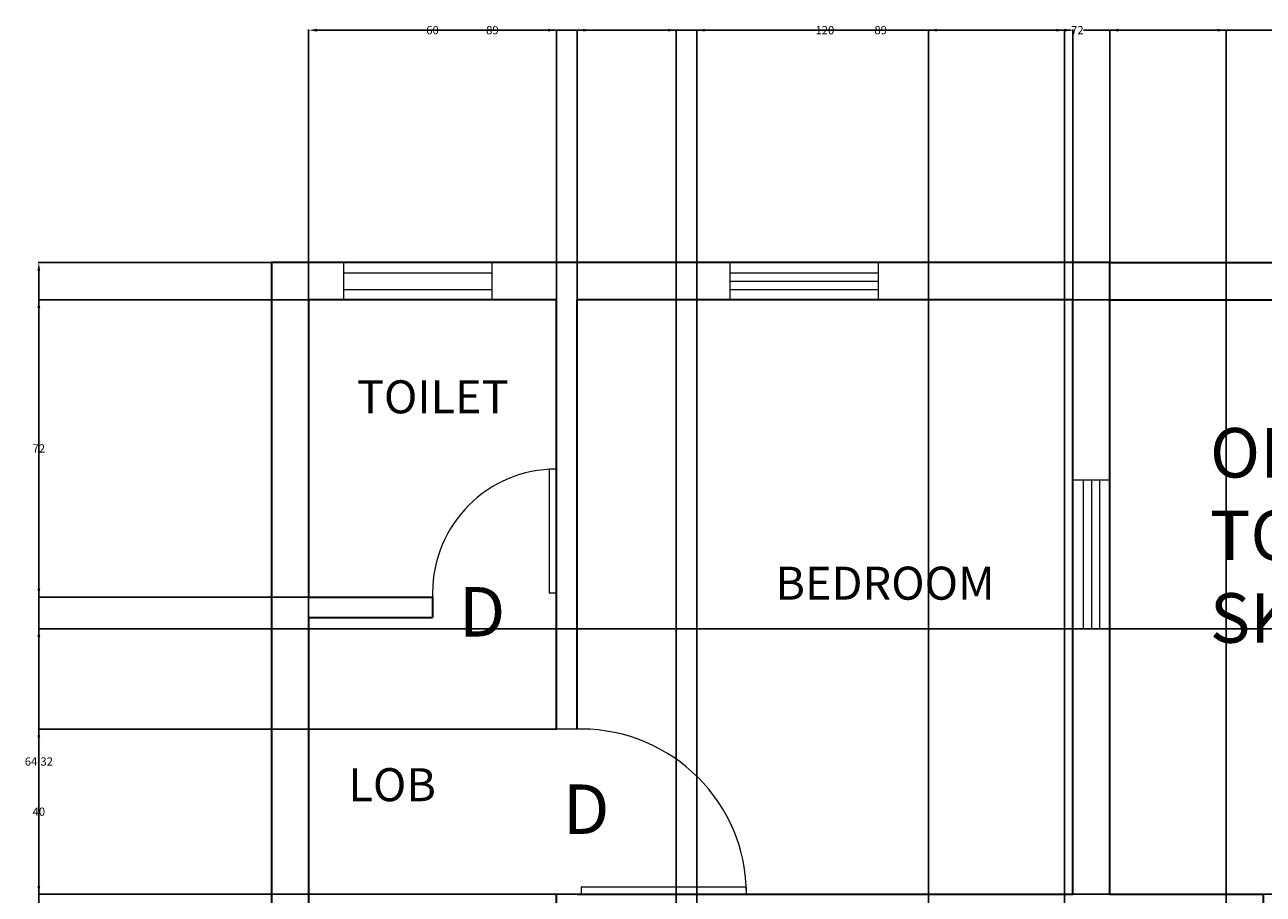
# Model space of a CAD drawing. Units: inches. Extents: x 190 to 836, y -241 to 999.
# Tile 7 of 9: x 191 to 491, y 789 to 999. Entities that reach past the tile are written whole.
import ezdxf

# ---------------------------------------------------------------- set-up
doc = ezdxf.new("R2010")
doc.units = ezdxf.units.IN
doc.header["$MEASUREMENT"] = 0
for name, color, linetype, lineweight in [('A-ANNO-DIMS', 2, 'Continuous', 18), ('A-ANNO-TEXT', 7, 'Continuous', 18), ('A-AREA-IDEN', 7, 'Continuous', 18), ('A-DOOR', 3, 'Continuous', 18), ('A-GLAZ', 4, 'Continuous', 18), ('A-WALL', 7, 'Continuous', 35)]:
    doc.layers.add(name, color=color, linetype=linetype, lineweight=lineweight)
doc.styles.get("Standard").update_dxf_attribs({"font": 'arial.ttf'})
doc.dimstyles.get("Standard").update_dxf_attribs({"dimtxt": 2, "dimasz": 2, "dimexe": 0.18, "dimexo": 0.0625, "dimgap": 0.09, "dimtad": 0, "dimtih": 1, "dimtoh": 1, "dimdec": 0, "dimzin": 0, "dimdsep": 46, "dimlunit": 3, "dimtxsty": 'Standard', "dimcen": 0.09, "dimadec": 0, "dimazin": 0, "dimtfac": 1, "dimtdec": 0, "dimtofl": 0, "dimtmove": 0, "dimatfit": 3, "dimfxl": 1, "dimtolj": 1, "dimtzin": 0, "dimarcsym": 0})

# ---------------------------------------------------------------- blocks, each defined once
blk = doc.blocks.new('*U2')
for p, q in [((0, 0), (0, 6)), ((40, 0), (40, 6))]:
    blk.add_line(p, q)
blk.add_lwpolyline([(0, 0), (0, -40), (1.75, -40), (1.75, 0)], close=True)
blk.add_arc((0, 0), 40, 270, 360)
blk = doc.blocks.new('*U3')
for p, q in [((-30, 0), (-30, -6)), ((0, 0), (0, -6))]:
    blk.add_line(p, q)
blk.add_lwpolyline([(0, 0), (0, 30), (-1.75, 30), (-1.75, 0)], close=True)
blk.add_arc((0, 0), 30, 90, 180)
blk = doc.blocks.new('WIN-36IN-9IN-3LINE')
for p, q in [((2.5, 36), (2.5, 0)), ((4.5, 36), (4.5, 0)), ((6.5, 36), (6.5, 0))]:
    blk.add_line(p, q)
blk.add_lwpolyline([(0, 0), (9, 0), (9, 36), (0, 36)], close=True)
blk = doc.blocks.new('WIN-36IN-9IN-2LINE')
for p, q in [((0, 6.5), (36, 6.5)), ((0, 2.5), (36, 2.5))]:
    blk.add_line(p, q)
blk.add_lwpolyline([(36, 0), (36, 9), (0, 9), (0, 0)], close=True)
blk = doc.blocks.new('*D17')
at = {"layer": 'A-ANNO-DIMS', "color": 0, "lineweight": -2, "transparency": 16777216}
for p, q in [((250.38, 941.53), (193.96, 941.53)), ((194.14, 939.53), (194.14, 380.14)), ((194.14, -181.47), (194.14, 377.92)), ((447.38, -183.47), (193.96, -183.47))]:
    blk.add_line(p, q, dxfattribs=at)
at = {"layer": 'A-ANNO-DIMS', "color": 0, "transparency": 16777216}
for points in [[(193.8, 939.53), (194.47, 939.53), (194.14, 941.53)], [(193.8, -181.47), (194.47, -181.47), (194.14, -183.47)]]:
    blk.add_solid(points, dxfattribs=at)
at = {"layer": 'Defpoints', "color": 0, "transparency": 16777216}
for p in [(194.14, 941.53), (250.44, 941.53), (447.44, -183.47)]:
    blk.add_point(p, dxfattribs=at)
at = {"layer": 'A-ANNO-DIMS', "color": 0, "transparency": 16777216, "insert": (194.14, 379.03), "char_height": 2, "attachment_point": 5}
blk.add_mtext('\\A1;1125', dxfattribs=at)
blk = doc.blocks.new('*D19')
at = {"layer": 'A-ANNO-DIMS', "color": 0, "lineweight": -2, "transparency": 16777216}
for p, q in [((453.44, 941.59), (453.44, 998.02)), ((455.44, 997.84), (511.24, 997.84)), ((571.44, 997.84), (515.64, 997.84)), ((573.44, 941.59), (573.44, 998.02))]:
    blk.add_line(p, q, dxfattribs=at)
at = {"layer": 'A-ANNO-DIMS', "color": 0, "transparency": 16777216}
for points in [[(455.44, 998.17), (455.44, 997.5), (453.44, 997.84)], [(571.44, 998.17), (571.44, 997.5), (573.44, 997.84)]]:
    blk.add_solid(points, dxfattribs=at)
at = {"layer": 'Defpoints', "color": 0, "transparency": 16777216}
for p in [(573.44, 997.84), (453.44, 941.53), (573.44, 941.53)]:
    blk.add_point(p, dxfattribs=at)
at = {"layer": 'A-ANNO-DIMS', "color": 0, "transparency": 16777216, "insert": (513.44, 997.84), "char_height": 2, "attachment_point": 5}
blk.add_mtext('\\A1;120', dxfattribs=at)
blk = doc.blocks.new('*D22')
at = {"layer": 'A-ANNO-DIMS', "color": 0, "lineweight": -2, "transparency": 16777216}
for p, q in [((259.44, 932.59), (259.44, 998.02)), ((261.44, 997.84), (287.92, 997.84)), ((317.44, 997.84), (290.97, 997.84)), ((319.44, 932.59), (319.44, 998.02))]:
    blk.add_line(p, q, dxfattribs=at)
at = {"layer": 'A-ANNO-DIMS', "color": 0, "transparency": 16777216}
for points in [[(261.44, 998.17), (261.44, 997.5), (259.44, 997.84)], [(317.44, 998.17), (317.44, 997.5), (319.44, 997.84)]]:
    blk.add_solid(points, dxfattribs=at)
at = {"layer": 'Defpoints', "color": 0, "transparency": 16777216}
for p in [(319.44, 997.84), (259.44, 932.53), (319.44, 932.53)]:
    blk.add_point(p, dxfattribs=at)
at = {"layer": 'A-ANNO-DIMS', "color": 0, "transparency": 16777216, "insert": (289.44, 997.84), "char_height": 2, "attachment_point": 5}
blk.add_mtext('\\A1;60', dxfattribs=at)
blk = doc.blocks.new('*D23')
at = {"layer": 'A-ANNO-DIMS', "color": 0, "lineweight": -2, "transparency": 16777216}
for p, q in [((324.44, 932.59), (324.44, 998.02)), ((326.44, 997.84), (382.24, 997.84)), ((442.44, 997.84), (386.64, 997.84)), ((444.44, 932.59), (444.44, 998.02))]:
    blk.add_line(p, q, dxfattribs=at)
at = {"layer": 'A-ANNO-DIMS', "color": 0, "transparency": 16777216}
for points in [[(326.44, 998.17), (326.44, 997.5), (324.44, 997.84)], [(442.44, 998.17), (442.44, 997.5), (444.44, 997.84)]]:
    blk.add_solid(points, dxfattribs=at)
at = {"layer": 'Defpoints', "color": 0, "transparency": 16777216}
for p in [(444.44, 997.84), (324.44, 932.53), (444.44, 932.53)]:
    blk.add_point(p, dxfattribs=at)
at = {"layer": 'A-ANNO-DIMS', "color": 0, "transparency": 16777216, "insert": (384.44, 997.84), "char_height": 2, "attachment_point": 5}
blk.add_mtext('\\A1;120', dxfattribs=at)
blk = doc.blocks.new('*D24')
at = {"layer": 'A-ANNO-DIMS', "color": 0, "lineweight": -2, "transparency": 16777216}
for p, q in [((259.38, 932.53), (193.96, 932.53)), ((194.14, 930.53), (194.14, 897.63)), ((194.14, 862.53), (194.14, 895.44)), ((259.38, 860.53), (193.96, 860.53))]:
    blk.add_line(p, q, dxfattribs=at)
at = {"layer": 'A-ANNO-DIMS', "color": 0, "transparency": 16777216}
for points in [[(193.8, 930.53), (194.47, 930.53), (194.14, 932.53)], [(193.8, 862.53), (194.47, 862.53), (194.14, 860.53)]]:
    blk.add_solid(points, dxfattribs=at)
at = {"layer": 'Defpoints', "color": 0, "transparency": 16777216}
for p in [(194.14, 932.53), (259.44, 932.53), (259.44, 860.53)]:
    blk.add_point(p, dxfattribs=at)
at = {"layer": 'A-ANNO-DIMS', "color": 0, "transparency": 16777216, "insert": (194.14, 896.53), "char_height": 2, "attachment_point": 5}
blk.add_mtext('\\A1;72', dxfattribs=at)
blk = doc.blocks.new('*D25')
at = {"layer": 'A-ANNO-DIMS', "color": 0, "lineweight": -2, "transparency": 16777216}
for p, q in [((444.5, 932.53), (832.94, 932.53)), ((832.76, 930.53), (832.76, 861.63)), ((832.76, 790.53), (832.76, 859.44)), ((444.5, 788.53), (832.94, 788.53))]:
    blk.add_line(p, q, dxfattribs=at)
at = {"layer": 'A-ANNO-DIMS', "color": 0, "transparency": 16777216}
for points in [[(832.43, 930.53), (833.1, 930.53), (832.76, 932.53)], [(832.43, 790.53), (833.1, 790.53), (832.76, 788.53)]]:
    blk.add_solid(points, dxfattribs=at)
at = {"layer": 'Defpoints', "color": 0, "transparency": 16777216}
for p in [(444.44, 932.53), (832.76, 932.53), (444.44, 788.53)]:
    blk.add_point(p, dxfattribs=at)
at = {"layer": 'A-ANNO-DIMS', "color": 0, "transparency": 16777216, "insert": (832.76, 860.53), "char_height": 2, "attachment_point": 5}
blk.add_mtext('\\A1;144', dxfattribs=at)
blk = doc.blocks.new('*D26')
at = {"layer": 'A-ANNO-DIMS', "color": 0, "lineweight": -2, "transparency": 16777216}
for p, q in [((409.55, 683.59), (409.55, 998.02)), ((411.55, 997.84), (444.05, 997.84)), ((479.55, 997.84), (447.06, 997.84)), ((481.55, 683.59), (481.55, 998.02))]:
    blk.add_line(p, q, dxfattribs=at)
at = {"layer": 'A-ANNO-DIMS', "color": 0, "transparency": 16777216}
for points in [[(411.55, 998.17), (411.55, 997.5), (409.55, 997.84)], [(479.55, 998.17), (479.55, 997.5), (481.55, 997.84)]]:
    blk.add_solid(points, dxfattribs=at)
at = {"layer": 'Defpoints', "color": 0, "transparency": 16777216}
for p in [(481.55, 997.84), (409.55, 683.53), (481.55, 683.53)]:
    blk.add_point(p, dxfattribs=at)
at = {"layer": 'A-ANNO-DIMS', "color": 0, "transparency": 16777216, "insert": (445.55, 997.84), "char_height": 2, "attachment_point": 5}
blk.add_mtext('\\A1;72', dxfattribs=at)
blk = doc.blocks.new('*D32')
at = {"layer": 'A-ANNO-DIMS', "color": 0, "lineweight": -2, "transparency": 16777216}
for p, q in [((319.38, 828.53), (193.96, 828.53)), ((194.14, 826.53), (194.14, 809.64)), ((194.14, 790.53), (194.14, 807.42)), ((319.38, 788.53), (193.96, 788.53))]:
    blk.add_line(p, q, dxfattribs=at)
at = {"layer": 'A-ANNO-DIMS', "color": 0, "transparency": 16777216}
for points in [[(193.8, 826.53), (194.47, 826.53), (194.14, 828.53)], [(193.8, 790.53), (194.47, 790.53), (194.14, 788.53)]]:
    blk.add_solid(points, dxfattribs=at)
at = {"layer": 'Defpoints', "color": 0, "transparency": 16777216}
for p in [(194.14, 828.53), (319.44, 828.53), (319.44, 788.53)]:
    blk.add_point(p, dxfattribs=at)
at = {"layer": 'A-ANNO-DIMS', "color": 0, "transparency": 16777216, "insert": (194.14, 808.53), "char_height": 2, "attachment_point": 5}
blk.add_mtext('\\A1;40', dxfattribs=at)
blk = doc.blocks.new('*D35')
at = {"layer": 'A-ANNO-DIMS', "color": 0, "lineweight": -2, "transparency": 16777216}
for p, q in [((259.44, -8.41), (259.44, 998.02)), ((261.44, 997.84), (302.42, 997.84)), ((346.44, 997.84), (305.47, 997.84)), ((348.44, -8.41), (348.44, 998.02))]:
    blk.add_line(p, q, dxfattribs=at)
at = {"layer": 'A-ANNO-DIMS', "color": 0, "transparency": 16777216}
for points in [[(261.44, 998.17), (261.44, 997.5), (259.44, 997.84)], [(346.44, 998.17), (346.44, 997.5), (348.44, 997.84)]]:
    blk.add_solid(points, dxfattribs=at)
at = {"layer": 'Defpoints', "color": 0, "transparency": 16777216}
for p in [(348.44, 997.84), (259.44, -8.47), (348.44, -8.47)]:
    blk.add_point(p, dxfattribs=at)
at = {"layer": 'A-ANNO-DIMS', "color": 0, "transparency": 16777216, "insert": (303.94, 997.84), "char_height": 2, "attachment_point": 5}
blk.add_mtext('\\A1;89', dxfattribs=at)
blk = doc.blocks.new('*D36')
at = {"layer": 'A-ANNO-DIMS', "color": 0, "lineweight": -2, "transparency": 16777216}
for p, q in [((353.44, -8.41), (353.44, 998.02)), ((355.44, 997.84), (396.42, 997.84)), ((440.44, 997.84), (399.47, 997.84)), ((442.44, -8.41), (442.44, 998.02))]:
    blk.add_line(p, q, dxfattribs=at)
at = {"layer": 'A-ANNO-DIMS', "color": 0, "transparency": 16777216}
for points in [[(355.44, 998.17), (355.44, 997.5), (353.44, 997.84)], [(440.44, 998.17), (440.44, 997.5), (442.44, 997.84)]]:
    blk.add_solid(points, dxfattribs=at)
at = {"layer": 'Defpoints', "color": 0, "transparency": 16777216}
for p in [(442.44, 997.84), (353.44, -8.47), (442.44, -8.47)]:
    blk.add_point(p, dxfattribs=at)
at = {"layer": 'A-ANNO-DIMS', "color": 0, "transparency": 16777216, "insert": (397.94, 997.84), "char_height": 2, "attachment_point": 5}
blk.add_mtext('\\A1;89', dxfattribs=at)
blk = doc.blocks.new('*D52')
at = {"layer": 'A-ANNO-DIMS', "color": 0, "lineweight": -2, "transparency": 16777216}
for p, q in [((582.38, 852.85), (193.96, 852.85)), ((194.14, 850.85), (194.14, 821.8)), ((194.14, 790.53), (194.14, 819.58)), ((582.38, 788.53), (193.96, 788.53))]:
    blk.add_line(p, q, dxfattribs=at)
at = {"layer": 'A-ANNO-DIMS', "color": 0, "transparency": 16777216}
for points in [[(193.8, 850.85), (194.47, 850.85), (194.14, 852.85)], [(193.8, 790.53), (194.47, 790.53), (194.14, 788.53)]]:
    blk.add_solid(points, dxfattribs=at)
at = {"layer": 'Defpoints', "color": 0, "transparency": 16777216}
for p in [(582.44, 852.85), (194.14, 788.53), (582.44, 788.53)]:
    blk.add_point(p, dxfattribs=at)
at = {"layer": 'A-ANNO-DIMS', "color": 0, "transparency": 16777216, "insert": (194.14, 820.69), "char_height": 2, "attachment_point": 5}
blk.add_mtext('\\A1;64.32', dxfattribs=at)

msp = doc.modelspace()

# ---------------------------------------------------------------- linework, layer by layer
at = {"layer": 'A-WALL'}
for p, q in [((250.4421, 941.5313), (250.4421, 556.5313)), ((453.4421, 941.5313), (250.4421, 941.5313)), ((453.4421, 941.5313), (573.4421, 941.5313)), ((453.4421, 788.5313), (453.4421, 941.5313)), ((259.4421, 932.5313), (259.4421, 860.5313)), ((319.4421, 932.5313), (259.4421, 932.5313)), ((319.4421, 828.5313), (319.4421, 932.5313)), ((324.4421, 828.5313), (324.4421, 932.5313)), ((444.4421, 932.5313), (324.4421, 932.5313)), ((444.4421, 788.5313), (444.4421, 932.5313)), ((453.4421, 932.5313), (573.4421, 932.5313)), ((259.4421, 860.5313), (289.4421, 860.5313)), ((289.4421, 860.5313), (289.4421, 855.5313)), ((259.4421, 855.5313), (289.4421, 855.5313)), ((259.4421, 855.5313), (259.4421, 565.5313)), ((319.4421, 779.5313), (319.4421, 788.5313)), ((324.4421, 788.5313), (444.4421, 788.5313)), ((453.4421, 788.5313), (490.5536, 788.5313)), ((490.5536, 788.5313), (490.5536, 732.9119))]:
    msp.add_line(p, q, dxfattribs=at)

# ---------------------------------------------------------------- block references
at = {"layer": 'A-DOOR'}
msp.add_blockref('*U3', (319.4421, 861.5313), dxfattribs=at)
at = {"layer": 'A-DOOR', "rotation": 90}
msp.add_blockref('*U2', (325.4421, 788.5313), dxfattribs=at)
at = {"layer": 'A-GLAZ'}
for name, p in [('WIN-36IN-9IN-2LINE', (267.917, 932.531)), ('WIN-36IN-9IN-3LINE', (444.442, 852.851))]:
    msp.add_blockref(name, p, dxfattribs=at)
at = {"layer": 'A-GLAZ', "rotation": 90.00000000000075}
msp.add_blockref('WIN-36IN-9IN-3LINE', (397.4358, 932.5312), dxfattribs=at)

# ---------------------------------------------------------------- texts
at = {"layer": 'A-ANNO-TEXT', "char_height": 12, "attachment_point": 1}
for insert in [(295.807, 862.9464), (321.0209, 815.1248)]:
    msp.add_mtext_dynamic_manual_height_columns('D', width=8.765037, gutter_width=1, heights=[0], dxfattribs=dict(at, insert=insert))
at = {"layer": 'A-AREA-IDEN', "attachment_point": 1}
for s, width, insert, char_height in [('TOILET', 33.040256, (271.1436, 913.0231), 8), ('OPEN TO SKY', 38.023659, (477.6605, 901.4652), 12), ('BEDROOM', 33.040256, (372.4463, 867.8794), 8), ('LOB', 33.040256, (269.0822, 819.0683), 8)]:
    msp.add_mtext_dynamic_manual_height_columns(s, width=width, gutter_width=1, heights=[0], dxfattribs=dict(at, insert=insert, char_height=char_height))

# ---------------------------------------------------------------- dimensions: what is measured, and where the dimension line sits
at = {"layer": 'A-ANNO-DIMS'}
for base, p1, p2, picture, middle in [((319.4421, 997.8363), (259.4421, 932.5313), (319.4421, 932.5313), '*D22', (289.4421, 997.8363)), ((348.4421, 997.8363), (259.4421, -8.4687), (348.4421, -8.4687), '*D35', (303.9421, 997.8363)), ((444.4421, 997.8363), (324.4421, 932.5313), (444.4421, 932.5313), '*D23', (384.4421, 997.8363)), ((442.4421, 997.8363), (353.4421, -8.4687), (442.4421, -8.4687), '*D36', (397.9421, 997.8363)), ((481.5536, 997.8363), (409.5536, 683.5313), (481.5536, 683.5313), '*D26', (445.5536, 997.8363)), ((573.4421, 997.8363), (453.4421, 941.5313), (573.4421, 941.5313), '*D19', (513.4421, 997.8363))]:
    dim = msp.add_linear_dim(base=base, p1=p1, p2=p2, dimstyle='Standard', override={"dimdec": 0, "dimlfac": 1, "dimrnd": 0, "dimzin": 0, "dimdsep": 46, "dimlunit": 2}, dxfattribs=at)
    dim.commit()
    dim.dimension.update_dxf_attribs({"geometry": picture, "text_midpoint": middle})
for base, p1, p2, override, picture, middle in [((194.1371, 941.5313), (447.4421, -183.4687), (250.4421, 941.5313), {"dimdec": 0, "dimlfac": 1, "dimrnd": 0, "dimzin": 0, "dimdsep": 46, "dimlunit": 2}, '*D17', (194.1371, 379.0313)), ((194.1371, 932.5313), (259.4421, 860.5313), (259.4421, 932.5313), {"dimdec": 0, "dimlfac": 1, "dimrnd": 0, "dimzin": 0, "dimdsep": 46, "dimlunit": 2}, '*D24', (194.1371, 896.5313)), ((832.7634, 932.5313), (444.4421, 788.5313), (444.4421, 932.5313), {"dimdec": 0, "dimlfac": 1, "dimrnd": 0, "dimzin": 0, "dimdsep": 46, "dimlunit": 2}, '*D25', (832.7634, 860.5313)), ((194.1371, 788.5313), (582.4421, 852.851), (582.4421, 788.5313), {"dimdec": 2, "dimlfac": 1, "dimrnd": 0, "dimzin": 0, "dimdsep": 46, "dimlunit": 2}, '*D52', (194.1371, 820.6912)), ((194.1371, 828.5313), (319.4421, 788.5313), (319.4421, 828.5313), {"dimdec": 0, "dimlfac": 1, "dimrnd": 0, "dimzin": 0, "dimdsep": 46, "dimlunit": 2}, '*D32', (194.1371, 808.5313))]:
    dim = msp.add_linear_dim(base=base, p1=p1, p2=p2, angle=90, dimstyle='Standard', override=override, dxfattribs=at)
    dim.commit()
    dim.dimension.update_dxf_attribs({"geometry": picture, "text_midpoint": middle})

doc.saveas('drawing.dxf')
